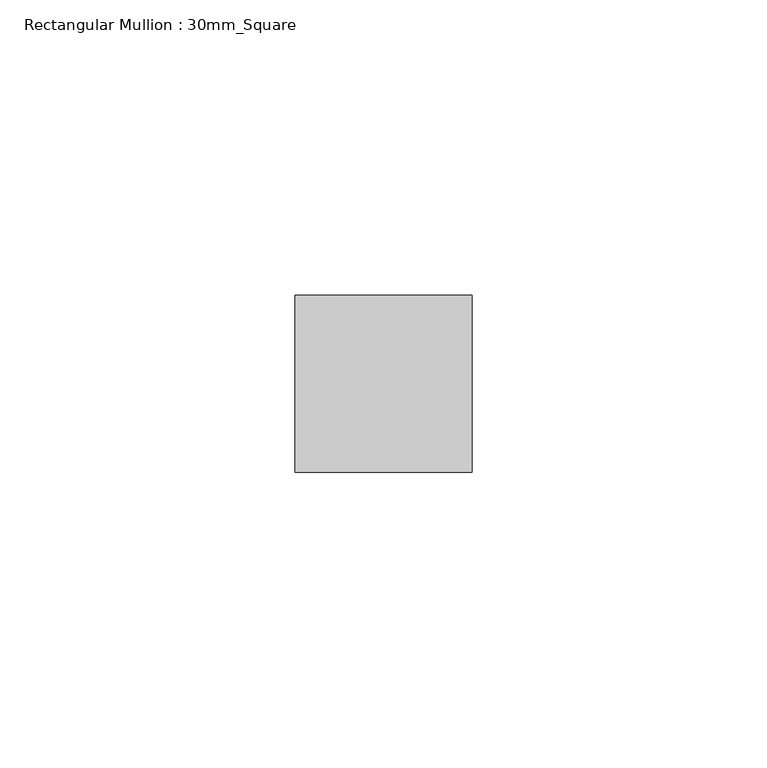
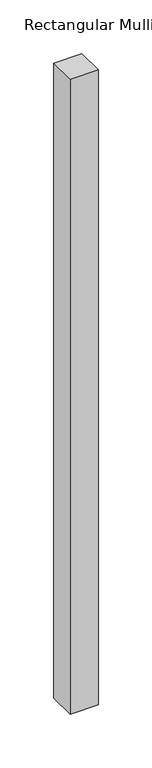
"""IFC4 building model written with IfcOpenShell, lengths in millimetres: member geometry, Rectangular Mullion : 30mm_Square."""

from ifc_helpers import new_model, si_unit, frame, origin, place, context, project, spatial, polyline, outline, extrude, source, transform, mapped, element, save


def rectangular_mullion_30mm_square_9902f449(model_context):
    return source(origin(), model_context, "Body", "SweptSolid", [
        extrude(outline(polyline([(0.0, 15.0), (0.0, -15.0), (-30.0, -15.0), (-30.0, 15.0), (0.0, 15.0)])), frame((0.0, 0.0, -719.4534873), z_axis=(0.0, 0.0, 1.0), x_axis=(1.0, 0.0, 0.0)), (0.0, 0.0, 1.0), 719.4534873),
    ])


if __name__ == "__main__":
    model = new_model("IFC4")
    model_context = context("Model", 3, world=origin())
    ifc_project = project(units=[si_unit("LENGTHUNIT", "METRE", prefix="MILLI")], contexts=[model_context])
    site = spatial("IfcSite", under=ifc_project)
    building = spatial("IfcBuilding", under=site)
    placement = place(None, origin())
    rectangular_mullion_30mm_square_shape = rectangular_mullion_30mm_square_9902f449(model_context)
    element("IfcMember", 1, ObjectType="Rectangular Mullion : 30mm_Square", at=placement, inside=building, context=model_context, shape_type="MappedRepresentation", body=[
        mapped(rectangular_mullion_30mm_square_shape, transform((0.0, 0.0, 0.0), x_axis=(1.0, 0.0, 0.0), y_axis=(0.0, 1.0, 0.0), z_axis=(0.0, 0.0, 1.0))),
    ])
    save(model, "model.ifc")

# Revit data of these elements
# Type "Rectangular Mullion : 30mm_Square"
#   Keynote = "H11"
#   built-in parameter 1007304 = 0.0984252 (stored number, unit not read)
#   built-in parameter 1007301 = 0.0492126 (stored number, unit not read)
#   built-in parameter 1007300 = 0.0492126 (stored number, unit not read)
# Element 1 (IfcMember, "Rectangular Mullion : 30mm_Square")
#   Materials on its faces: "Aluminium"
# Materials
#   "Aluminium": class "Metal", colour RGB 247 247 247, transparency 0, Description = "Aluminium 6061", Cost = 0
